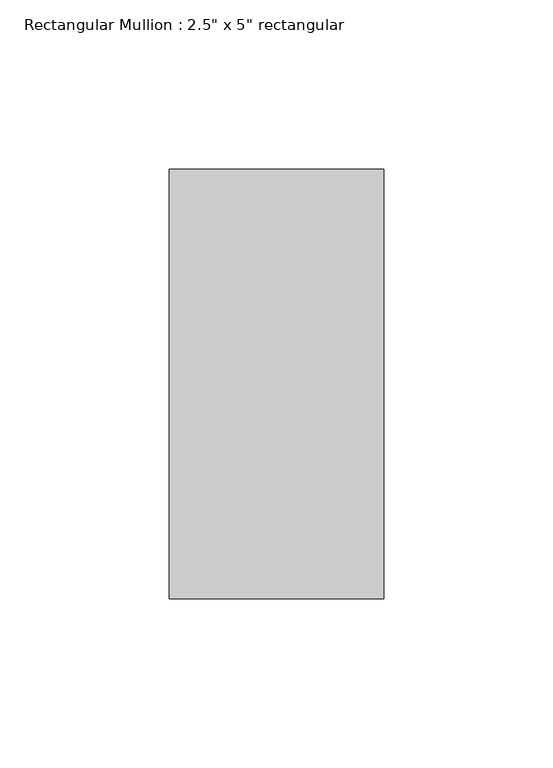
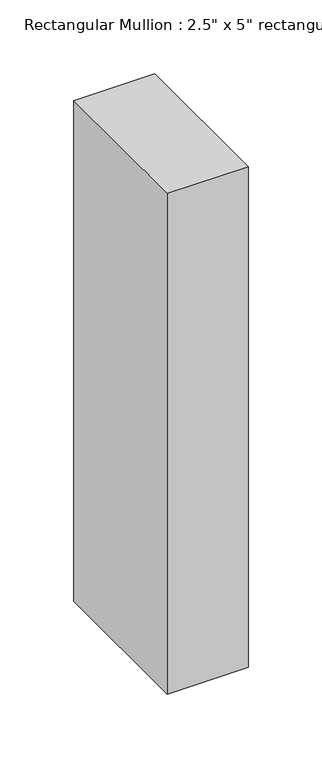
"""IFC4 building model written with IfcOpenShell, lengths in millimetres: member geometry."""

from ifc_helpers import new_model, si_unit, frame, origin, place, context, project, spatial, polyline, outline, extrude, source, transform, mapped, element, save


def member_471b44ca(model_context):
    return source(origin(), model_context, "Body", "SweptSolid", [
        extrude(outline(polyline([(31.75, 63.5), (31.75, -63.5), (-31.75, -63.5), (-31.75, 63.5), (31.75, 63.5)])), frame((0.0, 0.0, -414.8666667), z_axis=(0.0, 0.0, 1.0), x_axis=(1.0, 0.0, 0.0)), (0.0, 0.0, 1.0), 414.8666667),
    ])


if __name__ == "__main__":
    model = new_model("IFC4")
    model_context = context("Model", 3, world=origin())
    ifc_project = project(units=[si_unit("LENGTHUNIT", "METRE", prefix="MILLI")], contexts=[model_context])
    site = spatial("IfcSite", under=ifc_project)
    building = spatial("IfcBuilding", under=site)
    placement = place(None, origin())
    member_shape = member_471b44ca(model_context)
    element("IfcMember", 1, ObjectType="Rectangular Mullion : 2.5\" x 5\" rectangular", at=placement, inside=building, context=model_context, shape_type="MappedRepresentation", body=[
        mapped(member_shape, transform((0.0, 0.0, 0.0), x_axis=(1.0, 0.0, 0.0), y_axis=(0.0, 1.0, 0.0), z_axis=(0.0, 0.0, 1.0))),
    ])
    save(model, "model.ifc")

# Revit data of these elements
# Type "Rectangular Mullion : 2.5\" x 5\" rectangular"
#   built-in parameter 1007304 = 0.416667 (stored number, unit not read)
#   built-in parameter 1007301 = 0.104167 (stored number, unit not read)
#   built-in parameter 1007300 = 0.104167 (stored number, unit not read)
# Element 1 (IfcMember, "Rectangular Mullion : 2.5\" x 5\" rectangular")
#   Materials on its faces: "Aluminum"
# Materials
#   "Aluminum": class "Metal", colour RGB 247 247 247, transparency 0, Description = "Aluminum 6061", Cost = 0
